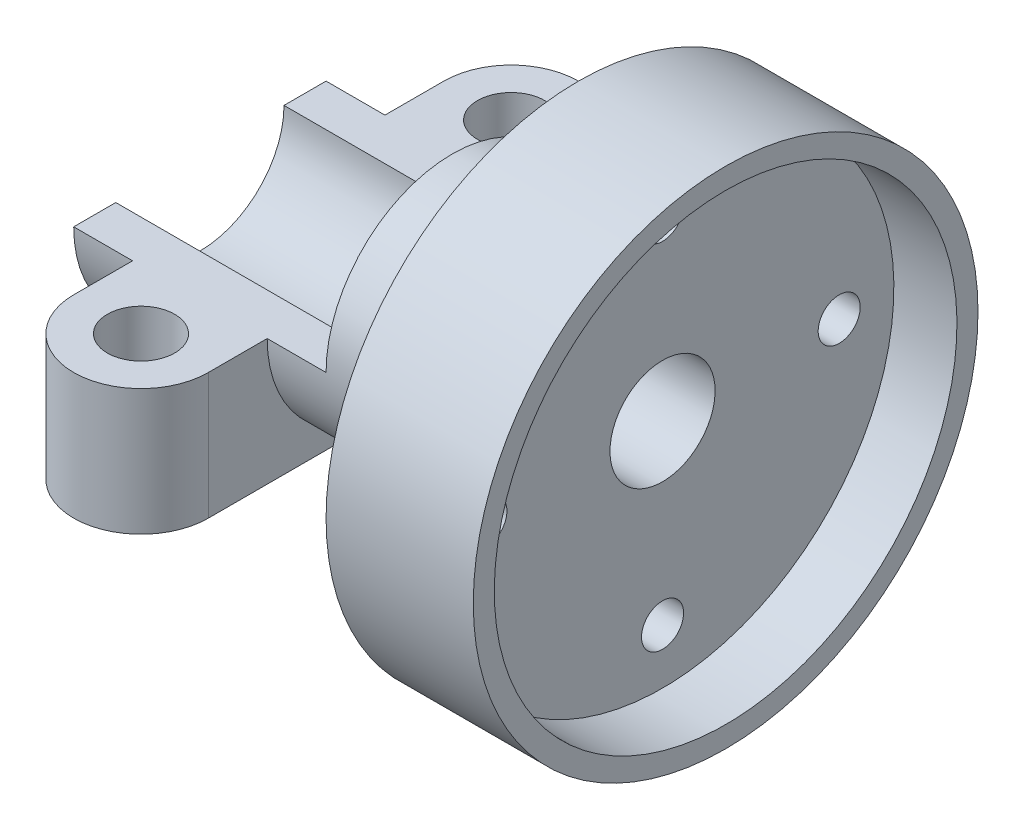
ISO-10303-21;
HEADER;
FILE_DESCRIPTION(('STEP AP214'),'2;1');
FILE_NAME('part.step','',(''),(''),'','','');
FILE_SCHEMA(('AUTOMOTIVE_DESIGN { 1 0 10303 214 1 1 1 1 }'));
ENDSEC;
DATA;
#1=APPLICATION_CONTEXT('core data for automotive mechanical design processes');
#2=APPLICATION_PROTOCOL_DEFINITION('international standard','automotive_design',2000,#1);
#3=PRODUCT_CONTEXT('',#1,'mechanical');
#4=PRODUCT('Part','Part','',(#3));
#5=PRODUCT_RELATED_PRODUCT_CATEGORY('part','',(#4));
#6=PRODUCT_DEFINITION_FORMATION('','',#4);
#7=PRODUCT_DEFINITION_CONTEXT('part definition',#1,'design');
#8=PRODUCT_DEFINITION('design','',#6,#7);
#9=PRODUCT_DEFINITION_SHAPE('','',#8);
#10=(LENGTH_UNIT() NAMED_UNIT(*) SI_UNIT(.MILLI.,.METRE.));
#11=(NAMED_UNIT(*) PLANE_ANGLE_UNIT() SI_UNIT($,.RADIAN.));
#12=(NAMED_UNIT(*) SI_UNIT($,.STERADIAN.) SOLID_ANGLE_UNIT());
#13=UNCERTAINTY_MEASURE_WITH_UNIT(LENGTH_MEASURE(1.E-05),#10,'distance_accuracy_value','');
#14=(GEOMETRIC_REPRESENTATION_CONTEXT(3) GLOBAL_UNCERTAINTY_ASSIGNED_CONTEXT((#13)) GLOBAL_UNIT_ASSIGNED_CONTEXT((#10,
#11,#12)) REPRESENTATION_CONTEXT('',''));
#15=CARTESIAN_POINT('',(0.,0.,0.));
#16=DIRECTION('',(0.,0.,1.));
#17=DIRECTION('',(1.,0.,0.));
#18=AXIS2_PLACEMENT_3D('',#15,#16,#17);
#19=CARTESIAN_POINT('',(-125.,0.,20.));
#20=DIRECTION('',(0.,-1.,0.));
#21=DIRECTION('',(1.,0.,0.));
#22=AXIS2_PLACEMENT_3D('',#19,#20,#21);
#23=PLANE('',#22);
#24=CARTESIAN_POINT('',(-95.,0.,44.));
#25=DIRECTION('',(0.,1.,0.));
#26=DIRECTION('',(-1.,0.,0.));
#27=AXIS2_PLACEMENT_3D('',#24,#25,#26);
#28=CIRCLE('',#27,8.);
#29=CARTESIAN_POINT('',(-103.,0.,44.));
#30=VERTEX_POINT('',#29);
#31=EDGE_CURVE('E312',#30,#30,#28,.T.);
#32=ORIENTED_EDGE('',*,*,#31,.F.);
#33=EDGE_LOOP('',(#32));
#34=FACE_BOUND('',#33,.T.);
#35=DIRECTION('',(0.,0.,-1.));
#36=VECTOR('',#35,1.);
#37=CARTESIAN_POINT('',(-65.,0.,20.));
#38=LINE('',#37,#36);
#39=CARTESIAN_POINT('',(-65.,0.,30.));
#40=VERTEX_POINT('',#39);
#41=CARTESIAN_POINT('',(-65.,0.,20.));
#42=VERTEX_POINT('',#41);
#43=EDGE_CURVE('E200',#40,#42,#38,.T.);
#44=ORIENTED_EDGE('',*,*,#43,.T.);
#45=DIRECTION('',(1.,0.,0.));
#46=VECTOR('',#45,1.);
#47=CARTESIAN_POINT('',(-125.,0.,20.));
#48=LINE('',#47,#46);
#49=CARTESIAN_POINT('',(-125.,0.,20.));
#50=VERTEX_POINT('',#49);
#51=EDGE_CURVE('E211',#50,#42,#48,.T.);
#52=ORIENTED_EDGE('',*,*,#51,.F.);
#53=DIRECTION('',(0.,0.,-1.));
#54=VECTOR('',#53,1.);
#55=CARTESIAN_POINT('',(-125.,0.,20.));
#56=LINE('',#55,#54);
#57=CARTESIAN_POINT('',(-125.,0.,30.));
#58=VERTEX_POINT('',#57);
#59=EDGE_CURVE('E192',#58,#50,#56,.T.);
#60=ORIENTED_EDGE('',*,*,#59,.F.);
#61=DIRECTION('',(1.,0.,0.));
#62=VECTOR('',#61,1.);
#63=CARTESIAN_POINT('',(-125.,0.,30.));
#64=LINE('',#63,#62);
#65=CARTESIAN_POINT('',(-111.,0.,30.));
#66=VERTEX_POINT('',#65);
#67=EDGE_CURVE('E212',#58,#66,#64,.T.);
#68=ORIENTED_EDGE('',*,*,#67,.T.);
#69=DIRECTION('',(0.,0.,1.));
#70=VECTOR('',#69,1.);
#71=CARTESIAN_POINT('',(-111.,0.,44.));
#72=LINE('',#71,#70);
#73=CARTESIAN_POINT('',(-111.,0.,44.));
#74=VERTEX_POINT('',#73);
#75=EDGE_CURVE('E159',#66,#74,#72,.T.);
#76=ORIENTED_EDGE('',*,*,#75,.T.);
#77=CARTESIAN_POINT('',(-95.,0.,44.));
#78=DIRECTION('',(0.,1.,0.));
#79=DIRECTION('',(-1.,0.,0.));
#80=AXIS2_PLACEMENT_3D('',#77,#78,#79);
#81=CIRCLE('',#80,16.);
#82=CARTESIAN_POINT('',(-79.,0.,44.));
#83=VERTEX_POINT('',#82);
#84=EDGE_CURVE('E173',#74,#83,#81,.T.);
#85=ORIENTED_EDGE('',*,*,#84,.T.);
#86=DIRECTION('',(0.,0.,-1.));
#87=VECTOR('',#86,1.);
#88=CARTESIAN_POINT('',(-79.,0.,44.));
#89=LINE('',#88,#87);
#90=CARTESIAN_POINT('',(-79.,0.,30.));
#91=VERTEX_POINT('',#90);
#92=EDGE_CURVE('E135',#83,#91,#89,.T.);
#93=ORIENTED_EDGE('',*,*,#92,.T.);
#94=EDGE_CURVE('E213',#91,#40,#64,.T.);
#95=ORIENTED_EDGE('',*,*,#94,.T.);
#96=EDGE_LOOP('',(#44,#52,#60,#68,#76,#85,#93,#95));
#97=FACE_BOUND('',#96,.T.);
#98=ADVANCED_FACE('F44',(#34,#97),#23,.F.);
#99=CARTESIAN_POINT('',(0.,0.,0.));
#100=DIRECTION('',(1.,0.,0.));
#101=DIRECTION('',(0.,1.,0.));
#102=AXIS2_PLACEMENT_3D('',#99,#100,#101);
#103=CYLINDRICAL_SURFACE('',#102,30.);
#104=CARTESIAN_POINT('',(-111.,0.,0.));
#105=DIRECTION('',(-1.,0.,0.));
#106=DIRECTION('',(0.,-1.,0.));
#107=AXIS2_PLACEMENT_3D('',#104,#105,#106);
#108=CIRCLE('',#107,30.);
#109=CARTESIAN_POINT('',(-111.,-30.,0.));
#110=VERTEX_POINT('',#109);
#111=CARTESIAN_POINT('',(-111.,0.,-30.));
#112=VERTEX_POINT('',#111);
#113=EDGE_CURVE('E58',#110,#112,#108,.F.);
#114=ORIENTED_EDGE('',*,*,#113,.F.);
#115=EDGE_CURVE('E188',#66,#110,#108,.F.);
#116=ORIENTED_EDGE('',*,*,#115,.F.);
#117=ORIENTED_EDGE('',*,*,#67,.F.);
#118=CARTESIAN_POINT('',(-125.,0.,0.));
#119=DIRECTION('',(-1.,0.,0.));
#120=DIRECTION('',(0.,-1.,0.));
#121=AXIS2_PLACEMENT_3D('',#118,#119,#120);
#122=CIRCLE('',#121,30.);
#123=CARTESIAN_POINT('',(-125.,0.,-30.));
#124=VERTEX_POINT('',#123);
#125=EDGE_CURVE('E187',#124,#58,#122,.T.);
#126=ORIENTED_EDGE('',*,*,#125,.F.);
#127=DIRECTION('',(1.,0.,0.));
#128=VECTOR('',#127,1.);
#129=CARTESIAN_POINT('',(-125.,0.,-30.));
#130=LINE('',#129,#128);
#131=EDGE_CURVE('E210',#124,#112,#130,.T.);
#132=ORIENTED_EDGE('',*,*,#131,.T.);
#133=EDGE_LOOP('',(#114,#116,#117,#126,#132));
#134=FACE_BOUND('',#133,.T.);
#135=ADVANCED_FACE('F277',(#134),#103,.T.);
#136=CARTESIAN_POINT('',(0.,55.,0.));
#137=DIRECTION('',(1.,0.,0.));
#138=DIRECTION('',(0.,1.,0.));
#139=AXIS2_PLACEMENT_3D('',#136,#137,#138);
#140=PLANE('',#139);
#141=CARTESIAN_POINT('',(0.,0.,0.));
#142=DIRECTION('',(1.,0.,0.));
#143=DIRECTION('',(0.,1.,0.));
#144=AXIS2_PLACEMENT_3D('',#141,#142,#143);
#145=CIRCLE('',#144,60.);
#146=CARTESIAN_POINT('',(0.,60.,0.));
#147=VERTEX_POINT('',#146);
#148=EDGE_CURVE('E11',#147,#147,#145,.T.);
#149=ORIENTED_EDGE('',*,*,#148,.T.);
#150=EDGE_LOOP('',(#149));
#151=FACE_BOUND('',#150,.T.);
#152=CARTESIAN_POINT('',(0.,0.,0.));
#153=DIRECTION('',(1.,0.,0.));
#154=DIRECTION('',(0.,1.,0.));
#155=AXIS2_PLACEMENT_3D('',#152,#153,#154);
#156=CIRCLE('',#155,55.);
#157=CARTESIAN_POINT('',(0.,55.,0.));
#158=VERTEX_POINT('',#157);
#159=EDGE_CURVE('E222',#158,#158,#156,.T.);
#160=ORIENTED_EDGE('',*,*,#159,.F.);
#161=EDGE_LOOP('',(#160));
#162=FACE_BOUND('',#161,.T.);
#163=ADVANCED_FACE('F50',(#151,#162),#140,.T.);
#164=CARTESIAN_POINT('',(0.,0.,0.));
#165=DIRECTION('',(1.,0.,0.));
#166=DIRECTION('',(0.,1.,0.));
#167=AXIS2_PLACEMENT_3D('',#164,#165,#166);
#168=CYLINDRICAL_SURFACE('',#167,60.);
#169=CARTESIAN_POINT('',(-35.,0.,0.));
#170=DIRECTION('',(1.,0.,0.));
#171=DIRECTION('',(0.,1.,0.));
#172=AXIS2_PLACEMENT_3D('',#169,#170,#171);
#173=CIRCLE('',#172,60.);
#174=CARTESIAN_POINT('',(-35.,60.,0.));
#175=VERTEX_POINT('',#174);
#176=EDGE_CURVE('E52',#175,#175,#173,.T.);
#177=ORIENTED_EDGE('',*,*,#176,.T.);
#178=EDGE_LOOP('',(#177));
#179=FACE_BOUND('',#178,.T.);
#180=ORIENTED_EDGE('',*,*,#148,.F.);
#181=EDGE_LOOP('',(#180));
#182=FACE_BOUND('',#181,.T.);
#183=ADVANCED_FACE('F261',(#179,#182),#168,.T.);
#184=CARTESIAN_POINT('',(-35.,60.,0.));
#185=DIRECTION('',(-1.,0.,0.));
#186=DIRECTION('',(0.,-1.,0.));
#187=AXIS2_PLACEMENT_3D('',#184,#185,#186);
#188=PLANE('',#187);
#189=CARTESIAN_POINT('',(-35.,0.,42.));
#190=DIRECTION('',(-1.,0.,0.));
#191=DIRECTION('',(0.,-1.,0.));
#192=AXIS2_PLACEMENT_3D('',#189,#190,#191);
#193=CIRCLE('',#192,5.);
#194=CARTESIAN_POINT('',(-35.,-4.99999999999999,42.));
#195=VERTEX_POINT('',#194);
#196=EDGE_CURVE('E217',#195,#195,#193,.T.);
#197=ORIENTED_EDGE('',*,*,#196,.F.);
#198=EDGE_LOOP('',(#197));
#199=FACE_BOUND('',#198,.T.);
#200=CARTESIAN_POINT('',(-35.,-42.,-1.46642216231412E-13));
#201=DIRECTION('',(-1.,0.,0.));
#202=DIRECTION('',(0.,-1.,0.));
#203=AXIS2_PLACEMENT_3D('',#200,#201,#202);
#204=CIRCLE('',#203,5.);
#205=CARTESIAN_POINT('',(-35.,-47.,-1.46642216231412E-13));
#206=VERTEX_POINT('',#205);
#207=EDGE_CURVE('E223',#206,#206,#204,.T.);
#208=ORIENTED_EDGE('',*,*,#207,.F.);
#209=EDGE_LOOP('',(#208));
#210=FACE_BOUND('',#209,.T.);
#211=CARTESIAN_POINT('',(-35.,0.,-42.));
#212=DIRECTION('',(-1.,0.,0.));
#213=DIRECTION('',(0.,-1.,0.));
#214=AXIS2_PLACEMENT_3D('',#211,#212,#213);
#215=CIRCLE('',#214,4.99999999999991);
#216=CARTESIAN_POINT('',(-35.,-4.99999999999991,-42.));
#217=VERTEX_POINT('',#216);
#218=EDGE_CURVE('E232',#217,#217,#215,.T.);
#219=ORIENTED_EDGE('',*,*,#218,.F.);
#220=EDGE_LOOP('',(#219));
#221=FACE_BOUND('',#220,.T.);
#222=CARTESIAN_POINT('',(-35.,42.,4.39926648694235E-13));
#223=DIRECTION('',(-1.,0.,0.));
#224=DIRECTION('',(0.,-1.,0.));
#225=AXIS2_PLACEMENT_3D('',#222,#223,#224);
#226=CIRCLE('',#225,5.);
#227=CARTESIAN_POINT('',(-35.,37.,4.39926648694235E-13));
#228=VERTEX_POINT('',#227);
#229=EDGE_CURVE('E240',#228,#228,#226,.T.);
#230=ORIENTED_EDGE('',*,*,#229,.F.);
#231=EDGE_LOOP('',(#230));
#232=FACE_BOUND('',#231,.T.);
#233=CARTESIAN_POINT('',(-35.,0.,0.));
#234=DIRECTION('',(1.,0.,0.));
#235=DIRECTION('',(0.,1.,0.));
#236=AXIS2_PLACEMENT_3D('',#233,#234,#235);
#237=CIRCLE('',#236,30.);
#238=CARTESIAN_POINT('',(-35.,30.,0.));
#239=VERTEX_POINT('',#238);
#240=EDGE_CURVE('E258',#239,#239,#237,.T.);
#241=ORIENTED_EDGE('',*,*,#240,.T.);
#242=EDGE_LOOP('',(#241));
#243=FACE_BOUND('',#242,.T.);
#244=ORIENTED_EDGE('',*,*,#176,.F.);
#245=EDGE_LOOP('',(#244));
#246=FACE_BOUND('',#245,.T.);
#247=ADVANCED_FACE('F262',(#199,#210,#221,#232,#243,#246),#188,.T.);
#248=CARTESIAN_POINT('',(-79.,0.,0.));
#249=DIRECTION('',(1.,0.,0.));
#250=DIRECTION('',(0.,1.,0.));
#251=AXIS2_PLACEMENT_3D('',#248,#249,#250);
#252=CIRCLE('',#251,30.);
#253=CARTESIAN_POINT('',(-79.,0.,-30.));
#254=VERTEX_POINT('',#253);
#255=CARTESIAN_POINT('',(-79.,-30.,0.));
#256=VERTEX_POINT('',#255);
#257=EDGE_CURVE('E183',#254,#256,#252,.F.);
#258=ORIENTED_EDGE('',*,*,#257,.F.);
#259=CARTESIAN_POINT('',(-65.,0.,-30.));
#260=VERTEX_POINT('',#259);
#261=EDGE_CURVE('E196',#254,#260,#130,.T.);
#262=ORIENTED_EDGE('',*,*,#261,.T.);
#263=CARTESIAN_POINT('',(-65.,0.,0.));
#264=DIRECTION('',(1.,0.,0.));
#265=DIRECTION('',(0.,1.,0.));
#266=AXIS2_PLACEMENT_3D('',#263,#264,#265);
#267=CIRCLE('',#266,30.);
#268=EDGE_CURVE('E251',#260,#40,#267,.T.);
#269=ORIENTED_EDGE('',*,*,#268,.T.);
#270=ORIENTED_EDGE('',*,*,#94,.F.);
#271=EDGE_CURVE('E70',#256,#91,#252,.F.);
#272=ORIENTED_EDGE('',*,*,#271,.F.);
#273=EDGE_LOOP('',(#258,#262,#269,#270,#272));
#274=FACE_BOUND('',#273,.T.);
#275=ORIENTED_EDGE('',*,*,#240,.F.);
#276=EDGE_LOOP('',(#275));
#277=FACE_BOUND('',#276,.T.);
#278=ADVANCED_FACE('F266',(#274,#277),#103,.T.);
#279=CARTESIAN_POINT('',(-65.,30.,0.));
#280=DIRECTION('',(-1.,0.,0.));
#281=DIRECTION('',(0.,-1.,0.));
#282=AXIS2_PLACEMENT_3D('',#279,#280,#281);
#283=PLANE('',#282);
#284=DIRECTION('',(0.,0.,-1.));
#285=VECTOR('',#284,1.);
#286=CARTESIAN_POINT('',(-65.,0.,-30.));
#287=LINE('',#286,#285);
#288=CARTESIAN_POINT('',(-65.,0.,-20.));
#289=VERTEX_POINT('',#288);
#290=EDGE_CURVE('E194',#289,#260,#287,.T.);
#291=ORIENTED_EDGE('',*,*,#290,.F.);
#292=CARTESIAN_POINT('',(-65.,0.,0.));
#293=DIRECTION('',(1.,0.,0.));
#294=DIRECTION('',(0.,-1.,0.));
#295=AXIS2_PLACEMENT_3D('',#292,#293,#294);
#296=CIRCLE('',#295,20.);
#297=EDGE_CURVE('E205',#42,#289,#296,.T.);
#298=ORIENTED_EDGE('',*,*,#297,.F.);
#299=ORIENTED_EDGE('',*,*,#43,.F.);
#300=ORIENTED_EDGE('',*,*,#268,.F.);
#301=EDGE_LOOP('',(#291,#298,#299,#300));
#302=FACE_BOUND('',#301,.T.);
#303=CARTESIAN_POINT('',(-65.,0.,0.));
#304=DIRECTION('',(1.,0.,0.));
#305=DIRECTION('',(0.,1.,0.));
#306=AXIS2_PLACEMENT_3D('',#303,#304,#305);
#307=CIRCLE('',#306,12.5);
#308=CARTESIAN_POINT('',(-65.,12.5,0.));
#309=VERTEX_POINT('',#308);
#310=EDGE_CURVE('E248',#309,#309,#307,.T.);
#311=ORIENTED_EDGE('',*,*,#310,.T.);
#312=EDGE_LOOP('',(#311));
#313=FACE_BOUND('',#312,.T.);
#314=ADVANCED_FACE('F273',(#302,#313),#283,.T.);
#315=CARTESIAN_POINT('',(0.,0.,0.));
#316=DIRECTION('',(1.,0.,0.));
#317=DIRECTION('',(0.,1.,0.));
#318=AXIS2_PLACEMENT_3D('',#315,#316,#317);
#319=CYLINDRICAL_SURFACE('',#318,12.5);
#320=CARTESIAN_POINT('',(-15.,0.,0.));
#321=DIRECTION('',(1.,0.,0.));
#322=DIRECTION('',(0.,1.,0.));
#323=AXIS2_PLACEMENT_3D('',#320,#321,#322);
#324=CIRCLE('',#323,12.5);
#325=CARTESIAN_POINT('',(-15.,12.5,0.));
#326=VERTEX_POINT('',#325);
#327=EDGE_CURVE('E249',#326,#326,#324,.T.);
#328=ORIENTED_EDGE('',*,*,#327,.T.);
#329=EDGE_LOOP('',(#328));
#330=FACE_BOUND('',#329,.T.);
#331=ORIENTED_EDGE('',*,*,#310,.F.);
#332=EDGE_LOOP('',(#331));
#333=FACE_BOUND('',#332,.T.);
#334=ADVANCED_FACE('F472',(#330,#333),#319,.F.);
#335=CARTESIAN_POINT('',(-15.,12.5,0.));
#336=DIRECTION('',(1.,0.,0.));
#337=DIRECTION('',(0.,1.,0.));
#338=AXIS2_PLACEMENT_3D('',#335,#336,#337);
#339=PLANE('',#338);
#340=CARTESIAN_POINT('',(-15.,0.,42.));
#341=DIRECTION('',(1.,0.,0.));
#342=DIRECTION('',(0.,1.,0.));
#343=AXIS2_PLACEMENT_3D('',#340,#341,#342);
#344=CIRCLE('',#343,5.);
#345=CARTESIAN_POINT('',(-15.,-5.,42.));
#346=VERTEX_POINT('',#345);
#347=EDGE_CURVE('E225',#346,#346,#344,.F.);
#348=ORIENTED_EDGE('',*,*,#347,.T.);
#349=EDGE_LOOP('',(#348));
#350=FACE_BOUND('',#349,.T.);
#351=CARTESIAN_POINT('',(-15.,-42.,-1.46642216231412E-13));
#352=DIRECTION('',(1.,0.,0.));
#353=DIRECTION('',(0.,1.,0.));
#354=AXIS2_PLACEMENT_3D('',#351,#352,#353);
#355=CIRCLE('',#354,5.);
#356=CARTESIAN_POINT('',(-15.,-47.,-1.46642216231412E-13));
#357=VERTEX_POINT('',#356);
#358=EDGE_CURVE('E227',#357,#357,#355,.F.);
#359=ORIENTED_EDGE('',*,*,#358,.T.);
#360=EDGE_LOOP('',(#359));
#361=FACE_BOUND('',#360,.T.);
#362=CARTESIAN_POINT('',(-15.,0.,-42.));
#363=DIRECTION('',(1.,0.,0.));
#364=DIRECTION('',(0.,1.,0.));
#365=AXIS2_PLACEMENT_3D('',#362,#363,#364);
#366=CIRCLE('',#365,4.99999999999991);
#367=CARTESIAN_POINT('',(-15.,-4.99999999999991,-42.));
#368=VERTEX_POINT('',#367);
#369=EDGE_CURVE('E231',#368,#368,#366,.F.);
#370=ORIENTED_EDGE('',*,*,#369,.T.);
#371=EDGE_LOOP('',(#370));
#372=FACE_BOUND('',#371,.T.);
#373=CARTESIAN_POINT('',(-15.,42.,4.39926648694235E-13));
#374=DIRECTION('',(1.,0.,0.));
#375=DIRECTION('',(0.,1.,0.));
#376=AXIS2_PLACEMENT_3D('',#373,#374,#375);
#377=CIRCLE('',#376,5.);
#378=CARTESIAN_POINT('',(-15.,37.,4.39926648694235E-13));
#379=VERTEX_POINT('',#378);
#380=EDGE_CURVE('E220',#379,#379,#377,.F.);
#381=ORIENTED_EDGE('',*,*,#380,.T.);
#382=EDGE_LOOP('',(#381));
#383=FACE_BOUND('',#382,.T.);
#384=CARTESIAN_POINT('',(-15.,0.,0.));
#385=DIRECTION('',(1.,0.,0.));
#386=DIRECTION('',(0.,1.,0.));
#387=AXIS2_PLACEMENT_3D('',#384,#385,#386);
#388=CIRCLE('',#387,55.);
#389=CARTESIAN_POINT('',(-15.,55.,0.));
#390=VERTEX_POINT('',#389);
#391=EDGE_CURVE('E245',#390,#390,#388,.T.);
#392=ORIENTED_EDGE('',*,*,#391,.T.);
#393=EDGE_LOOP('',(#392));
#394=FACE_BOUND('',#393,.T.);
#395=ORIENTED_EDGE('',*,*,#327,.F.);
#396=EDGE_LOOP('',(#395));
#397=FACE_BOUND('',#396,.T.);
#398=ADVANCED_FACE('F480',(#350,#361,#372,#383,#394,#397),#339,.T.);
#399=CARTESIAN_POINT('',(0.,0.,0.));
#400=DIRECTION('',(1.,0.,0.));
#401=DIRECTION('',(0.,1.,0.));
#402=AXIS2_PLACEMENT_3D('',#399,#400,#401);
#403=CYLINDRICAL_SURFACE('',#402,55.);
#404=ORIENTED_EDGE('',*,*,#159,.T.);
#405=EDGE_LOOP('',(#404));
#406=FACE_BOUND('',#405,.T.);
#407=ORIENTED_EDGE('',*,*,#391,.F.);
#408=EDGE_LOOP('',(#407));
#409=FACE_BOUND('',#408,.T.);
#410=ADVANCED_FACE('F491',(#406,#409),#403,.F.);
#411=CARTESIAN_POINT('',(0.00100000000001488,42.,4.39926648694235E-13));
#412=DIRECTION('',(-1.,0.,0.));
#413=DIRECTION('',(0.,-1.,0.));
#414=AXIS2_PLACEMENT_3D('',#411,#412,#413);
#415=CYLINDRICAL_SURFACE('',#414,5.);
#416=CARTESIAN_POINT('',(-15.,37.,4.39926648694235E-13));
#417=CARTESIAN_POINT('',(-15.2083333333333,37.,4.39926648694235E-13));
#418=CARTESIAN_POINT('',(-15.4166666666667,37.,4.39926648694235E-13));
#419=CARTESIAN_POINT('',(-15.8333333333333,37.,4.39926648694235E-13));
#420=CARTESIAN_POINT('',(-16.0416666666667,37.,4.39926648694235E-13));
#421=CARTESIAN_POINT('',(-16.4583333333333,37.,4.39926648694235E-13));
#422=CARTESIAN_POINT('',(-16.6666666666667,37.,4.39926648694235E-13));
#423=CARTESIAN_POINT('',(-17.0833333333333,37.,4.39926648694235E-13));
#424=CARTESIAN_POINT('',(-17.2916666666667,37.,4.39926648694235E-13));
#425=CARTESIAN_POINT('',(-17.7083333333333,37.,4.39926648694235E-13));
#426=CARTESIAN_POINT('',(-17.9166666666667,37.,4.39926648694235E-13));
#427=CARTESIAN_POINT('',(-18.3333333333333,37.,4.39926648694235E-13));
#428=CARTESIAN_POINT('',(-18.5416666666667,37.,4.39926648694235E-13));
#429=CARTESIAN_POINT('',(-18.9583333333333,37.,4.39926648694235E-13));
#430=CARTESIAN_POINT('',(-19.1666666666667,37.,4.39926648694235E-13));
#431=CARTESIAN_POINT('',(-19.5833333333333,37.,4.39926648694235E-13));
#432=CARTESIAN_POINT('',(-19.7916666666667,37.,4.39926648694235E-13));
#433=CARTESIAN_POINT('',(-20.2083333333333,37.,4.39926648694235E-13));
#434=CARTESIAN_POINT('',(-20.4166666666667,37.,4.39926648694235E-13));
#435=CARTESIAN_POINT('',(-20.8333333333333,37.,4.39926648694235E-13));
#436=CARTESIAN_POINT('',(-21.0416666666667,37.,4.39926648694235E-13));
#437=CARTESIAN_POINT('',(-21.4583333333333,37.,4.39926648694235E-13));
#438=CARTESIAN_POINT('',(-21.6666666666667,37.,4.39926648694235E-13));
#439=CARTESIAN_POINT('',(-22.0833333333333,37.,4.39926648694235E-13));
#440=CARTESIAN_POINT('',(-22.2916666666667,37.,4.39926648694235E-13));
#441=CARTESIAN_POINT('',(-22.7083333333333,37.,4.39926648694235E-13));
#442=CARTESIAN_POINT('',(-22.9166666666667,37.,4.39926648694235E-13));
#443=CARTESIAN_POINT('',(-23.3333333333333,37.,4.39926648694235E-13));
#444=CARTESIAN_POINT('',(-23.5416666666667,37.,4.39926648694235E-13));
#445=CARTESIAN_POINT('',(-23.9583333333333,37.,4.39926648694235E-13));
#446=CARTESIAN_POINT('',(-24.1666666666667,37.,4.39926648694235E-13));
#447=CARTESIAN_POINT('',(-24.5833333333333,37.,4.39926648694235E-13));
#448=CARTESIAN_POINT('',(-24.7916666666667,37.,4.39926648694235E-13));
#449=CARTESIAN_POINT('',(-25.2083333333333,37.,4.39926648694235E-13));
#450=CARTESIAN_POINT('',(-25.4166666666667,37.,4.39926648694235E-13));
#451=CARTESIAN_POINT('',(-25.8333333333333,37.,4.39926648694235E-13));
#452=CARTESIAN_POINT('',(-26.0416666666667,37.,4.39926648694235E-13));
#453=CARTESIAN_POINT('',(-26.4583333333333,37.,4.39926648694235E-13));
#454=CARTESIAN_POINT('',(-26.6666666666667,37.,4.39926648694235E-13));
#455=CARTESIAN_POINT('',(-27.0833333333333,37.,4.39926648694235E-13));
#456=CARTESIAN_POINT('',(-27.2916666666667,37.,4.39926648694235E-13));
#457=CARTESIAN_POINT('',(-27.7083333333333,37.,4.39926648694235E-13));
#458=CARTESIAN_POINT('',(-27.9166666666667,37.,4.39926648694235E-13));
#459=CARTESIAN_POINT('',(-28.3333333333333,37.,4.39926648694235E-13));
#460=CARTESIAN_POINT('',(-28.5416666666667,37.,4.39926648694235E-13));
#461=CARTESIAN_POINT('',(-28.9583333333333,37.,4.39926648694235E-13));
#462=CARTESIAN_POINT('',(-29.1666666666667,37.,4.39926648694235E-13));
#463=CARTESIAN_POINT('',(-29.5833333333333,37.,4.39926648694235E-13));
#464=CARTESIAN_POINT('',(-29.7916666666667,37.,4.39926648694235E-13));
#465=CARTESIAN_POINT('',(-30.2083333333333,37.,4.39926648694235E-13));
#466=CARTESIAN_POINT('',(-30.4166666666667,37.,4.39926648694235E-13));
#467=CARTESIAN_POINT('',(-30.8333333333333,37.,4.39926648694235E-13));
#468=CARTESIAN_POINT('',(-31.0416666666667,37.,4.39926648694235E-13));
#469=CARTESIAN_POINT('',(-31.4583333333333,37.,4.39926648694235E-13));
#470=CARTESIAN_POINT('',(-31.6666666666667,37.,4.39926648694235E-13));
#471=CARTESIAN_POINT('',(-32.0833333333333,37.,4.39926648694235E-13));
#472=CARTESIAN_POINT('',(-32.2916666666667,37.,4.39926648694235E-13));
#473=CARTESIAN_POINT('',(-32.7083333333333,37.,4.39926648694235E-13));
#474=CARTESIAN_POINT('',(-32.9166666666667,37.,4.39926648694235E-13));
#475=CARTESIAN_POINT('',(-33.3333333333333,37.,4.39926648694235E-13));
#476=CARTESIAN_POINT('',(-33.5416666666667,37.,4.39926648694235E-13));
#477=CARTESIAN_POINT('',(-33.9583333333333,37.,4.39926648694235E-13));
#478=CARTESIAN_POINT('',(-34.1666666666667,37.,4.39926648694235E-13));
#479=CARTESIAN_POINT('',(-34.5833333333333,37.,4.39926648694235E-13));
#480=CARTESIAN_POINT('',(-34.7916666666667,37.,4.39926648694235E-13));
#481=CARTESIAN_POINT('',(-35.,37.,4.39926648694235E-13));
#482=B_SPLINE_CURVE_WITH_KNOTS('',3,(#416,#417,#418,#419,#420,#421,#422,#423,#424,#425,#426,
#427,#428,#429,#430,#431,#432,#433,#434,#435,#436,#437,#438,#439,#440,#441,#442,#443,#444,#445,
#446,#447,#448,#449,#450,#451,#452,#453,#454,#455,#456,#457,#458,#459,#460,#461,#462,#463,#464,
#465,#466,#467,#468,#469,#470,#471,#472,#473,#474,#475,#476,#477,#478,#479,#480,#481),
.UNSPECIFIED.,.F.,.F.,(4,2,2,2,2,2,2,2,2,2,2,2,2,2,2,2,2,2,2,2,2,2,2,2,2,2,2,2,2,2,2,2,4),(0.,
0.624999999999999,1.25,1.875,2.5,3.125,3.75,4.375,5.,5.625,6.25,6.875,7.5,8.125,8.75,9.375,10.,
10.625,11.25,11.875,12.5,13.125,13.75,14.375,15.,15.625,16.25,16.875,17.5,18.125,18.75,19.375,
20.),.UNSPECIFIED.);
#483=EDGE_CURVE('BSEAM486',#379,#228,#482,.T.);
#484=ORIENTED_EDGE('',*,*,#380,.F.);
#485=ORIENTED_EDGE('',*,*,#229,.T.);
#486=ORIENTED_EDGE('',*,*,#483,.T.);
#487=ORIENTED_EDGE('',*,*,#483,.F.);
#488=EDGE_LOOP('',(#484,#486,#485,#487));
#489=FACE_BOUND('',#488,.T.);
#490=ADVANCED_FACE('F486',(#489),#415,.F.);
#491=CARTESIAN_POINT('',(0.00100000000000794,0.,-42.));
#492=DIRECTION('',(-1.,0.,0.));
#493=DIRECTION('',(0.,-1.,0.));
#494=AXIS2_PLACEMENT_3D('',#491,#492,#493);
#495=CYLINDRICAL_SURFACE('',#494,4.99999999999991);
#496=CARTESIAN_POINT('',(-15.,-4.99999999999991,-42.));
#497=CARTESIAN_POINT('',(-15.2083333333333,-4.99999999999991,-42.));
#498=CARTESIAN_POINT('',(-15.4166666666667,-4.99999999999991,-42.));
#499=CARTESIAN_POINT('',(-15.8333333333333,-4.99999999999991,-42.));
#500=CARTESIAN_POINT('',(-16.0416666666667,-4.99999999999991,-42.));
#501=CARTESIAN_POINT('',(-16.4583333333333,-4.99999999999991,-42.));
#502=CARTESIAN_POINT('',(-16.6666666666667,-4.99999999999991,-42.));
#503=CARTESIAN_POINT('',(-17.0833333333333,-4.99999999999991,-42.));
#504=CARTESIAN_POINT('',(-17.2916666666667,-4.99999999999991,-42.));
#505=CARTESIAN_POINT('',(-17.7083333333333,-4.99999999999991,-42.));
#506=CARTESIAN_POINT('',(-17.9166666666667,-4.99999999999991,-42.));
#507=CARTESIAN_POINT('',(-18.3333333333333,-4.99999999999991,-42.));
#508=CARTESIAN_POINT('',(-18.5416666666667,-4.99999999999991,-42.));
#509=CARTESIAN_POINT('',(-18.9583333333333,-4.99999999999991,-42.));
#510=CARTESIAN_POINT('',(-19.1666666666667,-4.99999999999991,-42.));
#511=CARTESIAN_POINT('',(-19.5833333333333,-4.99999999999991,-42.));
#512=CARTESIAN_POINT('',(-19.7916666666667,-4.99999999999991,-42.));
#513=CARTESIAN_POINT('',(-20.2083333333333,-4.99999999999991,-42.));
#514=CARTESIAN_POINT('',(-20.4166666666667,-4.99999999999991,-42.));
#515=CARTESIAN_POINT('',(-20.8333333333333,-4.99999999999991,-42.));
#516=CARTESIAN_POINT('',(-21.0416666666667,-4.99999999999991,-42.));
#517=CARTESIAN_POINT('',(-21.4583333333333,-4.99999999999991,-42.));
#518=CARTESIAN_POINT('',(-21.6666666666667,-4.99999999999991,-42.));
#519=CARTESIAN_POINT('',(-22.0833333333333,-4.99999999999991,-42.));
#520=CARTESIAN_POINT('',(-22.2916666666667,-4.99999999999991,-42.));
#521=CARTESIAN_POINT('',(-22.7083333333333,-4.99999999999991,-42.));
#522=CARTESIAN_POINT('',(-22.9166666666667,-4.99999999999991,-42.));
#523=CARTESIAN_POINT('',(-23.3333333333333,-4.99999999999991,-42.));
#524=CARTESIAN_POINT('',(-23.5416666666667,-4.99999999999991,-42.));
#525=CARTESIAN_POINT('',(-23.9583333333333,-4.99999999999991,-42.));
#526=CARTESIAN_POINT('',(-24.1666666666667,-4.99999999999991,-42.));
#527=CARTESIAN_POINT('',(-24.5833333333333,-4.99999999999991,-42.));
#528=CARTESIAN_POINT('',(-24.7916666666667,-4.99999999999991,-42.));
#529=CARTESIAN_POINT('',(-25.2083333333333,-4.99999999999991,-42.));
#530=CARTESIAN_POINT('',(-25.4166666666667,-4.99999999999991,-42.));
#531=CARTESIAN_POINT('',(-25.8333333333333,-4.99999999999991,-42.));
#532=CARTESIAN_POINT('',(-26.0416666666667,-4.99999999999991,-42.));
#533=CARTESIAN_POINT('',(-26.4583333333333,-4.99999999999991,-42.));
#534=CARTESIAN_POINT('',(-26.6666666666667,-4.99999999999991,-42.));
#535=CARTESIAN_POINT('',(-27.0833333333333,-4.99999999999991,-42.));
#536=CARTESIAN_POINT('',(-27.2916666666667,-4.99999999999991,-42.));
#537=CARTESIAN_POINT('',(-27.7083333333333,-4.99999999999991,-42.));
#538=CARTESIAN_POINT('',(-27.9166666666667,-4.99999999999991,-42.));
#539=CARTESIAN_POINT('',(-28.3333333333333,-4.99999999999991,-42.));
#540=CARTESIAN_POINT('',(-28.5416666666667,-4.99999999999991,-42.));
#541=CARTESIAN_POINT('',(-28.9583333333333,-4.99999999999991,-42.));
#542=CARTESIAN_POINT('',(-29.1666666666667,-4.99999999999991,-42.));
#543=CARTESIAN_POINT('',(-29.5833333333333,-4.99999999999991,-42.));
#544=CARTESIAN_POINT('',(-29.7916666666667,-4.99999999999991,-42.));
#545=CARTESIAN_POINT('',(-30.2083333333333,-4.99999999999991,-42.));
#546=CARTESIAN_POINT('',(-30.4166666666667,-4.99999999999991,-42.));
#547=CARTESIAN_POINT('',(-30.8333333333333,-4.99999999999991,-42.));
#548=CARTESIAN_POINT('',(-31.0416666666667,-4.99999999999991,-42.));
#549=CARTESIAN_POINT('',(-31.4583333333333,-4.99999999999991,-42.));
#550=CARTESIAN_POINT('',(-31.6666666666667,-4.99999999999991,-42.));
#551=CARTESIAN_POINT('',(-32.0833333333333,-4.99999999999991,-42.));
#552=CARTESIAN_POINT('',(-32.2916666666667,-4.99999999999991,-42.));
#553=CARTESIAN_POINT('',(-32.7083333333333,-4.99999999999991,-42.));
#554=CARTESIAN_POINT('',(-32.9166666666667,-4.99999999999991,-42.));
#555=CARTESIAN_POINT('',(-33.3333333333333,-4.99999999999991,-42.));
#556=CARTESIAN_POINT('',(-33.5416666666667,-4.99999999999991,-42.));
#557=CARTESIAN_POINT('',(-33.9583333333333,-4.99999999999991,-42.));
#558=CARTESIAN_POINT('',(-34.1666666666667,-4.99999999999991,-42.));
#559=CARTESIAN_POINT('',(-34.5833333333333,-4.99999999999991,-42.));
#560=CARTESIAN_POINT('',(-34.7916666666667,-4.99999999999991,-42.));
#561=CARTESIAN_POINT('',(-35.,-4.99999999999991,-42.));
#562=B_SPLINE_CURVE_WITH_KNOTS('',3,(#496,#497,#498,#499,#500,#501,#502,#503,#504,#505,#506,
#507,#508,#509,#510,#511,#512,#513,#514,#515,#516,#517,#518,#519,#520,#521,#522,#523,#524,#525,
#526,#527,#528,#529,#530,#531,#532,#533,#534,#535,#536,#537,#538,#539,#540,#541,#542,#543,#544,
#545,#546,#547,#548,#549,#550,#551,#552,#553,#554,#555,#556,#557,#558,#559,#560,#561),
.UNSPECIFIED.,.F.,.F.,(4,2,2,2,2,2,2,2,2,2,2,2,2,2,2,2,2,2,2,2,2,2,2,2,2,2,2,2,2,2,2,2,4),(0.,
0.624999999999999,1.25,1.875,2.5,3.125,3.75,4.375,5.,5.625,6.25,6.875,7.50000000000001,
8.12500000000001,8.75000000000001,9.37500000000001,10.,10.625,11.25,11.875,12.5,13.125,13.75,
14.375,15.,15.625,16.25,16.875,17.5,18.125,18.75,19.375,20.),.UNSPECIFIED.);
#563=EDGE_CURVE('BSEAM489',#368,#217,#562,.T.);
#564=ORIENTED_EDGE('',*,*,#369,.F.);
#565=ORIENTED_EDGE('',*,*,#218,.T.);
#566=ORIENTED_EDGE('',*,*,#563,.T.);
#567=ORIENTED_EDGE('',*,*,#563,.F.);
#568=EDGE_LOOP('',(#564,#566,#565,#567));
#569=FACE_BOUND('',#568,.T.);
#570=ADVANCED_FACE('F489',(#569),#495,.F.);
#571=CARTESIAN_POINT('',(0.001000000000001,-42.,-1.46642216231412E-13));
#572=DIRECTION('',(-1.,0.,0.));
#573=DIRECTION('',(0.,-1.,0.));
#574=AXIS2_PLACEMENT_3D('',#571,#572,#573);
#575=CYLINDRICAL_SURFACE('',#574,5.);
#576=CARTESIAN_POINT('',(-15.,-47.,-1.46642216231412E-13));
#577=CARTESIAN_POINT('',(-15.2083333333333,-47.,-1.46642216231412E-13));
#578=CARTESIAN_POINT('',(-15.4166666666667,-47.,-1.46642216231412E-13));
#579=CARTESIAN_POINT('',(-15.8333333333333,-47.,-1.46642216231412E-13));
#580=CARTESIAN_POINT('',(-16.0416666666667,-47.,-1.46642216231412E-13));
#581=CARTESIAN_POINT('',(-16.4583333333333,-47.,-1.46642216231412E-13));
#582=CARTESIAN_POINT('',(-16.6666666666667,-47.,-1.46642216231412E-13));
#583=CARTESIAN_POINT('',(-17.0833333333333,-47.,-1.46642216231412E-13));
#584=CARTESIAN_POINT('',(-17.2916666666667,-47.,-1.46642216231412E-13));
#585=CARTESIAN_POINT('',(-17.7083333333333,-47.,-1.46642216231412E-13));
#586=CARTESIAN_POINT('',(-17.9166666666667,-47.,-1.46642216231412E-13));
#587=CARTESIAN_POINT('',(-18.3333333333333,-47.,-1.46642216231412E-13));
#588=CARTESIAN_POINT('',(-18.5416666666667,-47.,-1.46642216231412E-13));
#589=CARTESIAN_POINT('',(-18.9583333333333,-47.,-1.46642216231412E-13));
#590=CARTESIAN_POINT('',(-19.1666666666667,-47.,-1.46642216231412E-13));
#591=CARTESIAN_POINT('',(-19.5833333333333,-47.,-1.46642216231412E-13));
#592=CARTESIAN_POINT('',(-19.7916666666667,-47.,-1.46642216231412E-13));
#593=CARTESIAN_POINT('',(-20.2083333333333,-47.,-1.46642216231412E-13));
#594=CARTESIAN_POINT('',(-20.4166666666667,-47.,-1.46642216231412E-13));
#595=CARTESIAN_POINT('',(-20.8333333333333,-47.,-1.46642216231412E-13));
#596=CARTESIAN_POINT('',(-21.0416666666667,-47.,-1.46642216231412E-13));
#597=CARTESIAN_POINT('',(-21.4583333333333,-47.,-1.46642216231412E-13));
#598=CARTESIAN_POINT('',(-21.6666666666667,-47.,-1.46642216231412E-13));
#599=CARTESIAN_POINT('',(-22.0833333333333,-47.,-1.46642216231412E-13));
#600=CARTESIAN_POINT('',(-22.2916666666667,-47.,-1.46642216231412E-13));
#601=CARTESIAN_POINT('',(-22.7083333333333,-47.,-1.46642216231412E-13));
#602=CARTESIAN_POINT('',(-22.9166666666667,-47.,-1.46642216231412E-13));
#603=CARTESIAN_POINT('',(-23.3333333333334,-47.,-1.46642216231412E-13));
#604=CARTESIAN_POINT('',(-23.5416666666667,-47.,-1.46642216231412E-13));
#605=CARTESIAN_POINT('',(-23.9583333333334,-47.,-1.46642216231412E-13));
#606=CARTESIAN_POINT('',(-24.1666666666667,-47.,-1.46642216231412E-13));
#607=CARTESIAN_POINT('',(-24.5833333333334,-47.,-1.46642216231412E-13));
#608=CARTESIAN_POINT('',(-24.7916666666667,-47.,-1.46642216231412E-13));
#609=CARTESIAN_POINT('',(-25.2083333333334,-47.,-1.46642216231412E-13));
#610=CARTESIAN_POINT('',(-25.4166666666667,-47.,-1.46642216231412E-13));
#611=CARTESIAN_POINT('',(-25.8333333333334,-47.,-1.46642216231412E-13));
#612=CARTESIAN_POINT('',(-26.0416666666667,-47.,-1.46642216231412E-13));
#613=CARTESIAN_POINT('',(-26.4583333333334,-47.,-1.46642216231412E-13));
#614=CARTESIAN_POINT('',(-26.6666666666667,-47.,-1.46642216231412E-13));
#615=CARTESIAN_POINT('',(-27.0833333333334,-47.,-1.46642216231412E-13));
#616=CARTESIAN_POINT('',(-27.2916666666667,-47.,-1.46642216231412E-13));
#617=CARTESIAN_POINT('',(-27.7083333333334,-47.,-1.46642216231412E-13));
#618=CARTESIAN_POINT('',(-27.9166666666667,-47.,-1.46642216231412E-13));
#619=CARTESIAN_POINT('',(-28.3333333333334,-47.,-1.46642216231412E-13));
#620=CARTESIAN_POINT('',(-28.5416666666667,-47.,-1.46642216231412E-13));
#621=CARTESIAN_POINT('',(-28.9583333333334,-47.,-1.46642216231412E-13));
#622=CARTESIAN_POINT('',(-29.1666666666667,-47.,-1.46642216231412E-13));
#623=CARTESIAN_POINT('',(-29.5833333333334,-47.,-1.46642216231412E-13));
#624=CARTESIAN_POINT('',(-29.7916666666667,-47.,-1.46642216231412E-13));
#625=CARTESIAN_POINT('',(-30.2083333333334,-47.,-1.46642216231412E-13));
#626=CARTESIAN_POINT('',(-30.4166666666667,-47.,-1.46642216231412E-13));
#627=CARTESIAN_POINT('',(-30.8333333333334,-47.,-1.46642216231412E-13));
#628=CARTESIAN_POINT('',(-31.0416666666667,-47.,-1.46642216231412E-13));
#629=CARTESIAN_POINT('',(-31.4583333333334,-47.,-1.46642216231412E-13));
#630=CARTESIAN_POINT('',(-31.6666666666667,-47.,-1.46642216231412E-13));
#631=CARTESIAN_POINT('',(-32.0833333333333,-47.,-1.46642216231412E-13));
#632=CARTESIAN_POINT('',(-32.2916666666667,-47.,-1.46642216231412E-13));
#633=CARTESIAN_POINT('',(-32.7083333333333,-47.,-1.46642216231412E-13));
#634=CARTESIAN_POINT('',(-32.9166666666667,-47.,-1.46642216231412E-13));
#635=CARTESIAN_POINT('',(-33.3333333333334,-47.,-1.46642216231412E-13));
#636=CARTESIAN_POINT('',(-33.5416666666667,-47.,-1.46642216231412E-13));
#637=CARTESIAN_POINT('',(-33.9583333333334,-47.,-1.46642216231412E-13));
#638=CARTESIAN_POINT('',(-34.1666666666667,-47.,-1.46642216231412E-13));
#639=CARTESIAN_POINT('',(-34.5833333333334,-47.,-1.46642216231412E-13));
#640=CARTESIAN_POINT('',(-34.7916666666667,-47.,-1.46642216231412E-13));
#641=CARTESIAN_POINT('',(-35.,-47.,-1.46642216231412E-13));
#642=B_SPLINE_CURVE_WITH_KNOTS('',3,(#576,#577,#578,#579,#580,#581,#582,#583,#584,#585,#586,
#587,#588,#589,#590,#591,#592,#593,#594,#595,#596,#597,#598,#599,#600,#601,#602,#603,#604,#605,
#606,#607,#608,#609,#610,#611,#612,#613,#614,#615,#616,#617,#618,#619,#620,#621,#622,#623,#624,
#625,#626,#627,#628,#629,#630,#631,#632,#633,#634,#635,#636,#637,#638,#639,#640,#641),
.UNSPECIFIED.,.F.,.F.,(4,2,2,2,2,2,2,2,2,2,2,2,2,2,2,2,2,2,2,2,2,2,2,2,2,2,2,2,2,2,2,2,4),(0.,
0.624999999999999,1.25,1.875,2.5,3.125,3.75,4.375,5.,5.625,6.25,6.875,7.50000000000001,
8.12500000000001,8.75000000000001,9.37500000000001,10.,10.625,11.25,11.875,12.5,13.125,13.75,
14.375,15.,15.625,16.25,16.875,17.5,18.125,18.75,19.375,20.),.UNSPECIFIED.);
#643=EDGE_CURVE('BSEAM305',#357,#206,#642,.T.);
#644=ORIENTED_EDGE('',*,*,#358,.F.);
#645=ORIENTED_EDGE('',*,*,#207,.T.);
#646=ORIENTED_EDGE('',*,*,#643,.T.);
#647=ORIENTED_EDGE('',*,*,#643,.F.);
#648=EDGE_LOOP('',(#644,#646,#645,#647));
#649=FACE_BOUND('',#648,.T.);
#650=ADVANCED_FACE('F305',(#649),#575,.F.);
#651=CARTESIAN_POINT('',(0.00100000000000794,0.,42.));
#652=DIRECTION('',(-1.,0.,0.));
#653=DIRECTION('',(0.,-1.,0.));
#654=AXIS2_PLACEMENT_3D('',#651,#652,#653);
#655=CYLINDRICAL_SURFACE('',#654,5.);
#656=CARTESIAN_POINT('',(-15.,-5.,42.));
#657=CARTESIAN_POINT('',(-15.2083333333333,-5.,42.));
#658=CARTESIAN_POINT('',(-15.4166666666667,-5.,42.));
#659=CARTESIAN_POINT('',(-15.8333333333333,-5.,42.));
#660=CARTESIAN_POINT('',(-16.0416666666667,-5.,42.));
#661=CARTESIAN_POINT('',(-16.4583333333333,-5.,42.));
#662=CARTESIAN_POINT('',(-16.6666666666667,-5.,42.));
#663=CARTESIAN_POINT('',(-17.0833333333333,-5.,42.));
#664=CARTESIAN_POINT('',(-17.2916666666667,-4.99999999999999,42.));
#665=CARTESIAN_POINT('',(-17.7083333333333,-4.99999999999999,42.));
#666=CARTESIAN_POINT('',(-17.9166666666667,-4.99999999999999,42.));
#667=CARTESIAN_POINT('',(-18.3333333333333,-4.99999999999999,42.));
#668=CARTESIAN_POINT('',(-18.5416666666667,-4.99999999999999,42.));
#669=CARTESIAN_POINT('',(-18.9583333333333,-4.99999999999999,42.));
#670=CARTESIAN_POINT('',(-19.1666666666667,-4.99999999999999,42.));
#671=CARTESIAN_POINT('',(-19.5833333333333,-4.99999999999999,42.));
#672=CARTESIAN_POINT('',(-19.7916666666667,-4.99999999999999,42.));
#673=CARTESIAN_POINT('',(-20.2083333333333,-4.99999999999999,42.));
#674=CARTESIAN_POINT('',(-20.4166666666667,-4.99999999999999,42.));
#675=CARTESIAN_POINT('',(-20.8333333333333,-4.99999999999999,42.));
#676=CARTESIAN_POINT('',(-21.0416666666667,-4.99999999999999,42.));
#677=CARTESIAN_POINT('',(-21.4583333333333,-4.99999999999999,42.));
#678=CARTESIAN_POINT('',(-21.6666666666667,-4.99999999999999,42.));
#679=CARTESIAN_POINT('',(-22.0833333333333,-4.99999999999999,42.));
#680=CARTESIAN_POINT('',(-22.2916666666667,-4.99999999999999,42.));
#681=CARTESIAN_POINT('',(-22.7083333333333,-4.99999999999999,42.));
#682=CARTESIAN_POINT('',(-22.9166666666667,-4.99999999999999,42.));
#683=CARTESIAN_POINT('',(-23.3333333333333,-4.99999999999999,42.));
#684=CARTESIAN_POINT('',(-23.5416666666667,-4.99999999999999,42.));
#685=CARTESIAN_POINT('',(-23.9583333333333,-4.99999999999999,42.));
#686=CARTESIAN_POINT('',(-24.1666666666667,-4.99999999999999,42.));
#687=CARTESIAN_POINT('',(-24.5833333333333,-4.99999999999999,42.));
#688=CARTESIAN_POINT('',(-24.7916666666667,-4.99999999999999,42.));
#689=CARTESIAN_POINT('',(-25.2083333333333,-4.99999999999999,42.));
#690=CARTESIAN_POINT('',(-25.4166666666667,-4.99999999999999,42.));
#691=CARTESIAN_POINT('',(-25.8333333333333,-4.99999999999999,42.));
#692=CARTESIAN_POINT('',(-26.0416666666667,-4.99999999999999,42.));
#693=CARTESIAN_POINT('',(-26.4583333333333,-4.99999999999999,42.));
#694=CARTESIAN_POINT('',(-26.6666666666667,-4.99999999999999,42.));
#695=CARTESIAN_POINT('',(-27.0833333333333,-4.99999999999999,42.));
#696=CARTESIAN_POINT('',(-27.2916666666667,-4.99999999999999,42.));
#697=CARTESIAN_POINT('',(-27.7083333333333,-4.99999999999999,42.));
#698=CARTESIAN_POINT('',(-27.9166666666667,-4.99999999999999,42.));
#699=CARTESIAN_POINT('',(-28.3333333333333,-4.99999999999999,42.));
#700=CARTESIAN_POINT('',(-28.5416666666667,-4.99999999999999,42.));
#701=CARTESIAN_POINT('',(-28.9583333333333,-4.99999999999999,42.));
#702=CARTESIAN_POINT('',(-29.1666666666667,-4.99999999999999,42.));
#703=CARTESIAN_POINT('',(-29.5833333333333,-4.99999999999999,42.));
#704=CARTESIAN_POINT('',(-29.7916666666667,-4.99999999999999,42.));
#705=CARTESIAN_POINT('',(-30.2083333333333,-4.99999999999999,42.));
#706=CARTESIAN_POINT('',(-30.4166666666667,-4.99999999999999,42.));
#707=CARTESIAN_POINT('',(-30.8333333333333,-4.99999999999999,42.));
#708=CARTESIAN_POINT('',(-31.0416666666667,-4.99999999999999,42.));
#709=CARTESIAN_POINT('',(-31.4583333333333,-4.99999999999999,42.));
#710=CARTESIAN_POINT('',(-31.6666666666667,-4.99999999999999,42.));
#711=CARTESIAN_POINT('',(-32.0833333333333,-4.99999999999999,42.));
#712=CARTESIAN_POINT('',(-32.2916666666667,-4.99999999999999,42.));
#713=CARTESIAN_POINT('',(-32.7083333333333,-4.99999999999999,42.));
#714=CARTESIAN_POINT('',(-32.9166666666667,-4.99999999999999,42.));
#715=CARTESIAN_POINT('',(-33.3333333333333,-4.99999999999999,42.));
#716=CARTESIAN_POINT('',(-33.5416666666667,-4.99999999999999,42.));
#717=CARTESIAN_POINT('',(-33.9583333333333,-4.99999999999999,42.));
#718=CARTESIAN_POINT('',(-34.1666666666667,-4.99999999999999,42.));
#719=CARTESIAN_POINT('',(-34.5833333333333,-4.99999999999999,42.));
#720=CARTESIAN_POINT('',(-34.7916666666667,-4.99999999999999,42.));
#721=CARTESIAN_POINT('',(-35.,-4.99999999999999,42.));
#722=B_SPLINE_CURVE_WITH_KNOTS('',3,(#656,#657,#658,#659,#660,#661,#662,#663,#664,#665,#666,
#667,#668,#669,#670,#671,#672,#673,#674,#675,#676,#677,#678,#679,#680,#681,#682,#683,#684,#685,
#686,#687,#688,#689,#690,#691,#692,#693,#694,#695,#696,#697,#698,#699,#700,#701,#702,#703,#704,
#705,#706,#707,#708,#709,#710,#711,#712,#713,#714,#715,#716,#717,#718,#719,#720,#721),
.UNSPECIFIED.,.F.,.F.,(4,2,2,2,2,2,2,2,2,2,2,2,2,2,2,2,2,2,2,2,2,2,2,2,2,2,2,2,2,2,2,2,4),(0.,
0.624999999999999,1.25,1.875,2.5,3.125,3.75,4.375,5.,5.625,6.25,6.875,7.50000000000001,
8.12500000000001,8.75000000000001,9.37500000000001,10.,10.625,11.25,11.875,12.5,13.125,13.75,
14.375,15.,15.625,16.25,16.875,17.5,18.125,18.75,19.375,20.),.UNSPECIFIED.);
#723=EDGE_CURVE('BSEAM294',#346,#195,#722,.T.);
#724=ORIENTED_EDGE('',*,*,#347,.F.);
#725=ORIENTED_EDGE('',*,*,#196,.T.);
#726=ORIENTED_EDGE('',*,*,#723,.T.);
#727=ORIENTED_EDGE('',*,*,#723,.F.);
#728=EDGE_LOOP('',(#724,#726,#725,#727));
#729=FACE_BOUND('',#728,.T.);
#730=ADVANCED_FACE('F294',(#729),#655,.F.);
#731=DIRECTION('',(1.,0.,0.));
#732=VECTOR('',#731,1.);
#733=CARTESIAN_POINT('',(-125.,0.,-20.));
#734=LINE('',#733,#732);
#735=CARTESIAN_POINT('',(-125.,0.,-20.));
#736=VERTEX_POINT('',#735);
#737=EDGE_CURVE('E207',#736,#289,#734,.T.);
#738=ORIENTED_EDGE('',*,*,#737,.T.);
#739=ORIENTED_EDGE('',*,*,#290,.T.);
#740=ORIENTED_EDGE('',*,*,#261,.F.);
#741=CARTESIAN_POINT('',(-79.,0.,-44.));
#742=VERTEX_POINT('',#741);
#743=EDGE_CURVE('E172',#254,#742,#89,.T.);
#744=ORIENTED_EDGE('',*,*,#743,.T.);
#745=CARTESIAN_POINT('',(-95.,0.,-44.));
#746=DIRECTION('',(0.,1.,0.));
#747=DIRECTION('',(-1.,0.,0.));
#748=AXIS2_PLACEMENT_3D('',#745,#746,#747);
#749=CIRCLE('',#748,16.);
#750=CARTESIAN_POINT('',(-111.,0.,-44.));
#751=VERTEX_POINT('',#750);
#752=EDGE_CURVE('E177',#742,#751,#749,.T.);
#753=ORIENTED_EDGE('',*,*,#752,.T.);
#754=EDGE_CURVE('E160',#751,#112,#72,.T.);
#755=ORIENTED_EDGE('',*,*,#754,.T.);
#756=ORIENTED_EDGE('',*,*,#131,.F.);
#757=DIRECTION('',(0.,0.,-1.));
#758=VECTOR('',#757,1.);
#759=CARTESIAN_POINT('',(-125.,0.,-30.));
#760=LINE('',#759,#758);
#761=EDGE_CURVE('E198',#736,#124,#760,.T.);
#762=ORIENTED_EDGE('',*,*,#761,.F.);
#763=EDGE_LOOP('',(#738,#739,#740,#744,#753,#755,#756,#762));
#764=FACE_BOUND('',#763,.T.);
#765=CARTESIAN_POINT('',(-95.,0.,-44.));
#766=DIRECTION('',(0.,1.,0.));
#767=DIRECTION('',(-1.,0.,0.));
#768=AXIS2_PLACEMENT_3D('',#765,#766,#767);
#769=CIRCLE('',#768,8.);
#770=CARTESIAN_POINT('',(-103.,0.,-44.));
#771=VERTEX_POINT('',#770);
#772=EDGE_CURVE('E162',#771,#771,#769,.T.);
#773=ORIENTED_EDGE('',*,*,#772,.F.);
#774=EDGE_LOOP('',(#773));
#775=FACE_BOUND('',#774,.T.);
#776=ADVANCED_FACE('F282',(#764,#775),#23,.F.);
#777=CARTESIAN_POINT('',(-125.,0.,0.));
#778=DIRECTION('',(1.,0.,0.));
#779=DIRECTION('',(0.,1.,0.));
#780=AXIS2_PLACEMENT_3D('',#777,#778,#779);
#781=CYLINDRICAL_SURFACE('',#780,20.);
#782=ORIENTED_EDGE('',*,*,#297,.T.);
#783=ORIENTED_EDGE('',*,*,#737,.F.);
#784=CARTESIAN_POINT('',(-125.,0.,0.));
#785=DIRECTION('',(1.,0.,0.));
#786=DIRECTION('',(0.,-1.,0.));
#787=AXIS2_PLACEMENT_3D('',#784,#785,#786);
#788=CIRCLE('',#787,20.);
#789=EDGE_CURVE('E191',#50,#736,#788,.T.);
#790=ORIENTED_EDGE('',*,*,#789,.F.);
#791=ORIENTED_EDGE('',*,*,#51,.T.);
#792=EDGE_LOOP('',(#782,#783,#790,#791));
#793=FACE_BOUND('',#792,.T.);
#794=ADVANCED_FACE('F291',(#793),#781,.F.);
#795=CARTESIAN_POINT('',(-125.,0.,0.));
#796=DIRECTION('',(-1.,0.,0.));
#797=DIRECTION('',(0.,-1.,0.));
#798=AXIS2_PLACEMENT_3D('',#795,#796,#797);
#799=PLANE('',#798);
#800=ORIENTED_EDGE('',*,*,#125,.T.);
#801=ORIENTED_EDGE('',*,*,#59,.T.);
#802=ORIENTED_EDGE('',*,*,#789,.T.);
#803=ORIENTED_EDGE('',*,*,#761,.T.);
#804=EDGE_LOOP('',(#800,#801,#802,#803));
#805=FACE_BOUND('',#804,.T.);
#806=ADVANCED_FACE('F296',(#805),#799,.T.);
#807=CARTESIAN_POINT('',(-95.,-30.,44.));
#808=DIRECTION('',(0.,1.,0.));
#809=DIRECTION('',(-1.,0.,0.));
#810=AXIS2_PLACEMENT_3D('',#807,#808,#809);
#811=PLANE('',#810);
#812=CARTESIAN_POINT('',(-95.,-30.,-44.));
#813=DIRECTION('',(0.,1.,0.));
#814=DIRECTION('',(-1.,0.,0.));
#815=AXIS2_PLACEMENT_3D('',#812,#813,#814);
#816=CIRCLE('',#815,8.);
#817=CARTESIAN_POINT('',(-103.,-30.,-44.));
#818=VERTEX_POINT('',#817);
#819=EDGE_CURVE('E175',#818,#818,#816,.T.);
#820=ORIENTED_EDGE('',*,*,#819,.T.);
#821=EDGE_LOOP('',(#820));
#822=FACE_BOUND('',#821,.T.);
#823=DIRECTION('',(0.,0.,-1.));
#824=VECTOR('',#823,1.);
#825=CARTESIAN_POINT('',(-79.,-30.,44.));
#826=LINE('',#825,#824);
#827=CARTESIAN_POINT('',(-79.,-30.,-44.));
#828=VERTEX_POINT('',#827);
#829=EDGE_CURVE('E147',#256,#828,#826,.T.);
#830=ORIENTED_EDGE('',*,*,#829,.F.);
#831=CARTESIAN_POINT('',(-79.,-30.,44.));
#832=VERTEX_POINT('',#831);
#833=EDGE_CURVE('E134',#832,#256,#826,.T.);
#834=ORIENTED_EDGE('',*,*,#833,.F.);
#835=CARTESIAN_POINT('',(-95.,-30.,44.));
#836=DIRECTION('',(0.,1.,0.));
#837=DIRECTION('',(-1.,0.,0.));
#838=AXIS2_PLACEMENT_3D('',#835,#836,#837);
#839=CIRCLE('',#838,16.);
#840=CARTESIAN_POINT('',(-111.,-30.,44.));
#841=VERTEX_POINT('',#840);
#842=EDGE_CURVE('E146',#841,#832,#839,.T.);
#843=ORIENTED_EDGE('',*,*,#842,.F.);
#844=DIRECTION('',(0.,0.,1.));
#845=VECTOR('',#844,1.);
#846=CARTESIAN_POINT('',(-111.,-30.,44.));
#847=LINE('',#846,#845);
#848=EDGE_CURVE('E169',#110,#841,#847,.T.);
#849=ORIENTED_EDGE('',*,*,#848,.F.);
#850=CARTESIAN_POINT('',(-111.,-30.,-44.));
#851=VERTEX_POINT('',#850);
#852=EDGE_CURVE('E138',#851,#110,#847,.T.);
#853=ORIENTED_EDGE('',*,*,#852,.F.);
#854=CARTESIAN_POINT('',(-95.,-30.,-44.));
#855=DIRECTION('',(0.,1.,0.));
#856=DIRECTION('',(-1.,0.,0.));
#857=AXIS2_PLACEMENT_3D('',#854,#855,#856);
#858=CIRCLE('',#857,16.);
#859=EDGE_CURVE('E151',#828,#851,#858,.T.);
#860=ORIENTED_EDGE('',*,*,#859,.F.);
#861=EDGE_LOOP('',(#830,#834,#843,#849,#853,#860));
#862=FACE_BOUND('',#861,.T.);
#863=CARTESIAN_POINT('',(-95.,-30.,44.));
#864=DIRECTION('',(0.,1.,0.));
#865=DIRECTION('',(-1.,0.,0.));
#866=AXIS2_PLACEMENT_3D('',#863,#864,#865);
#867=CIRCLE('',#866,8.);
#868=CARTESIAN_POINT('',(-103.,-30.,44.));
#869=VERTEX_POINT('',#868);
#870=EDGE_CURVE('E315',#869,#869,#867,.T.);
#871=ORIENTED_EDGE('',*,*,#870,.T.);
#872=EDGE_LOOP('',(#871));
#873=FACE_BOUND('',#872,.T.);
#874=ADVANCED_FACE('F144',(#822,#862,#873),#811,.F.);
#875=CARTESIAN_POINT('',(-111.,-30.,44.));
#876=DIRECTION('',(-1.,0.,0.));
#877=DIRECTION('',(0.,-1.,0.));
#878=AXIS2_PLACEMENT_3D('',#875,#876,#877);
#879=PLANE('',#878);
#880=ORIENTED_EDGE('',*,*,#852,.T.);
#881=ORIENTED_EDGE('',*,*,#113,.T.);
#882=ORIENTED_EDGE('',*,*,#754,.F.);
#883=DIRECTION('',(0.,1.,0.));
#884=VECTOR('',#883,1.);
#885=CARTESIAN_POINT('',(-111.,-30.,-44.));
#886=LINE('',#885,#884);
#887=EDGE_CURVE('E178',#851,#751,#886,.T.);
#888=ORIENTED_EDGE('',*,*,#887,.F.);
#889=EDGE_LOOP('',(#880,#881,#882,#888));
#890=FACE_BOUND('',#889,.T.);
#891=ADVANCED_FACE('F331',(#890),#879,.T.);
#892=CARTESIAN_POINT('',(-79.,-30.,44.));
#893=DIRECTION('',(1.,0.,0.));
#894=DIRECTION('',(0.,1.,0.));
#895=AXIS2_PLACEMENT_3D('',#892,#893,#894);
#896=PLANE('',#895);
#897=ORIENTED_EDGE('',*,*,#743,.F.);
#898=ORIENTED_EDGE('',*,*,#257,.T.);
#899=ORIENTED_EDGE('',*,*,#829,.T.);
#900=DIRECTION('',(0.,1.,0.));
#901=VECTOR('',#900,1.);
#902=CARTESIAN_POINT('',(-79.,-30.,-44.));
#903=LINE('',#902,#901);
#904=EDGE_CURVE('E136',#828,#742,#903,.T.);
#905=ORIENTED_EDGE('',*,*,#904,.T.);
#906=EDGE_LOOP('',(#897,#898,#899,#905));
#907=FACE_BOUND('',#906,.T.);
#908=ADVANCED_FACE('F347',(#907),#896,.T.);
#909=CARTESIAN_POINT('',(-95.,-30.,44.));
#910=DIRECTION('',(0.,1.,0.));
#911=DIRECTION('',(-1.,0.,0.));
#912=AXIS2_PLACEMENT_3D('',#909,#910,#911);
#913=CYLINDRICAL_SURFACE('',#912,16.);
#914=ORIENTED_EDGE('',*,*,#84,.F.);
#915=DIRECTION('',(0.,1.,0.));
#916=VECTOR('',#915,1.);
#917=CARTESIAN_POINT('',(-111.,-30.,44.));
#918=LINE('',#917,#916);
#919=EDGE_CURVE('E156',#841,#74,#918,.T.);
#920=ORIENTED_EDGE('',*,*,#919,.F.);
#921=ORIENTED_EDGE('',*,*,#842,.T.);
#922=DIRECTION('',(0.,1.,0.));
#923=VECTOR('',#922,1.);
#924=CARTESIAN_POINT('',(-79.,-30.,44.));
#925=LINE('',#924,#923);
#926=EDGE_CURVE('E129',#832,#83,#925,.T.);
#927=ORIENTED_EDGE('',*,*,#926,.T.);
#928=EDGE_LOOP('',(#914,#920,#921,#927));
#929=FACE_BOUND('',#928,.T.);
#930=ADVANCED_FACE('F152',(#929),#913,.T.);
#931=ORIENTED_EDGE('',*,*,#75,.F.);
#932=ORIENTED_EDGE('',*,*,#115,.T.);
#933=ORIENTED_EDGE('',*,*,#848,.T.);
#934=ORIENTED_EDGE('',*,*,#919,.T.);
#935=EDGE_LOOP('',(#931,#932,#933,#934));
#936=FACE_BOUND('',#935,.T.);
#937=ADVANCED_FACE('F338',(#936),#879,.T.);
#938=CARTESIAN_POINT('',(-95.,-30.,-44.));
#939=DIRECTION('',(0.,1.,0.));
#940=DIRECTION('',(-1.,0.,0.));
#941=AXIS2_PLACEMENT_3D('',#938,#939,#940);
#942=CYLINDRICAL_SURFACE('',#941,16.);
#943=ORIENTED_EDGE('',*,*,#752,.F.);
#944=ORIENTED_EDGE('',*,*,#904,.F.);
#945=ORIENTED_EDGE('',*,*,#859,.T.);
#946=ORIENTED_EDGE('',*,*,#887,.T.);
#947=EDGE_LOOP('',(#943,#944,#945,#946));
#948=FACE_BOUND('',#947,.T.);
#949=ADVANCED_FACE('F340',(#948),#942,.T.);
#950=ORIENTED_EDGE('',*,*,#833,.T.);
#951=ORIENTED_EDGE('',*,*,#271,.T.);
#952=ORIENTED_EDGE('',*,*,#92,.F.);
#953=ORIENTED_EDGE('',*,*,#926,.F.);
#954=EDGE_LOOP('',(#950,#951,#952,#953));
#955=FACE_BOUND('',#954,.T.);
#956=ADVANCED_FACE('F133',(#955),#896,.T.);
#957=CARTESIAN_POINT('',(-95.,-30.,-44.));
#958=DIRECTION('',(0.,1.,0.));
#959=DIRECTION('',(-1.,0.,0.));
#960=AXIS2_PLACEMENT_3D('',#957,#958,#959);
#961=CYLINDRICAL_SURFACE('',#960,8.);
#962=ORIENTED_EDGE('',*,*,#819,.F.);
#963=EDGE_LOOP('',(#962));
#964=FACE_BOUND('',#963,.T.);
#965=ORIENTED_EDGE('',*,*,#772,.T.);
#966=EDGE_LOOP('',(#965));
#967=FACE_BOUND('',#966,.T.);
#968=ADVANCED_FACE('F323',(#964,#967),#961,.F.);
#969=CARTESIAN_POINT('',(-95.,-30.,44.));
#970=DIRECTION('',(0.,1.,0.));
#971=DIRECTION('',(-1.,0.,0.));
#972=AXIS2_PLACEMENT_3D('',#969,#970,#971);
#973=CYLINDRICAL_SURFACE('',#972,8.);
#974=ORIENTED_EDGE('',*,*,#870,.F.);
#975=EDGE_LOOP('',(#974));
#976=FACE_BOUND('',#975,.T.);
#977=ORIENTED_EDGE('',*,*,#31,.T.);
#978=EDGE_LOOP('',(#977));
#979=FACE_BOUND('',#978,.T.);
#980=ADVANCED_FACE('F321',(#976,#979),#973,.F.);
#981=CLOSED_SHELL('',(#98,#135,#163,#183,#247,#278,#314,#334,#398,#410,#490,#570,#650,#730,#776,
#794,#806,#874,#891,#908,#930,#937,#949,#956,#968,#980));
#982=MANIFOLD_SOLID_BREP('B2',#981);
#983=ADVANCED_BREP_SHAPE_REPRESENTATION('',(#18,#982),#14);
#984=SHAPE_DEFINITION_REPRESENTATION(#9,#983);
ENDSEC;
END-ISO-10303-21;
